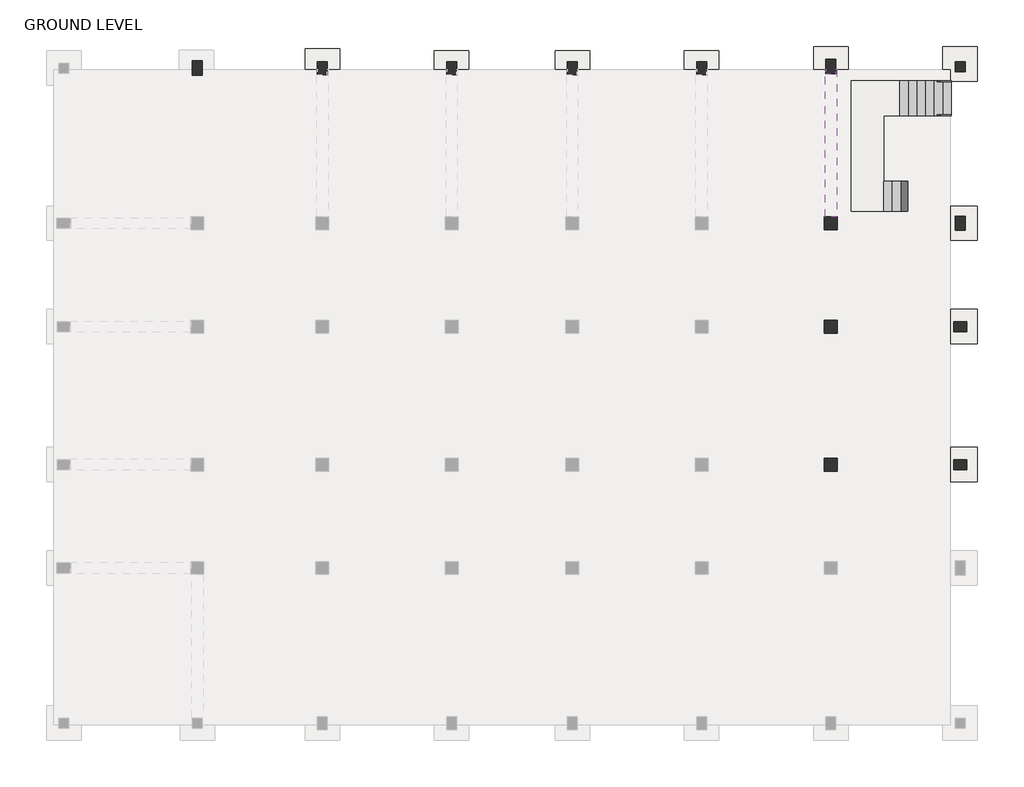
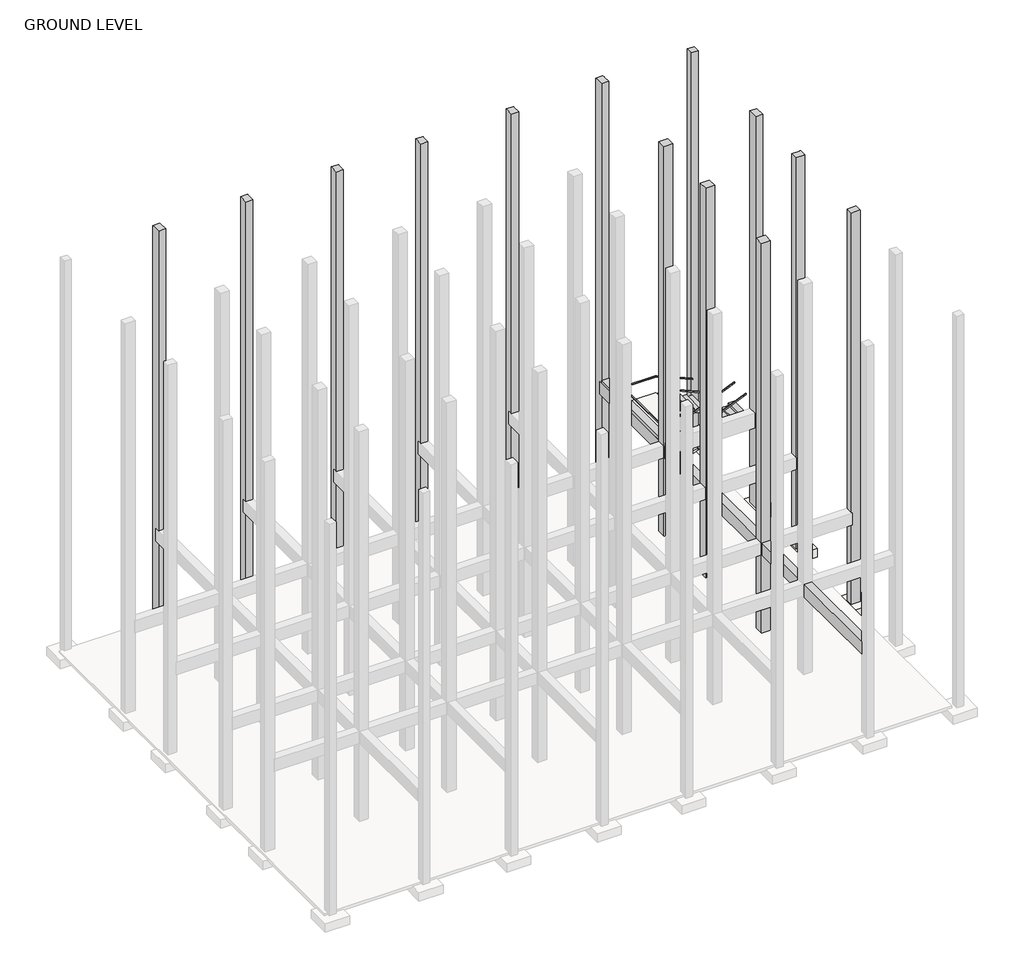
# One storey, part 3 of 3: 13 columns, 13 slabs, 2 railings, 2 stair flights, 1 beam.
"""IFC4 building model written with IfcOpenShell, lengths in millimetres."""

from ifc_helpers import new_model, si_unit, frame, origin, place, context, project, spatial, polyline, outline, extrude, faceted_brep, element, save

model = new_model("IFC4")

# Units and contexts
model_context = context("Model", 3, world=origin())
ifc_project = project(units=[si_unit("LENGTHUNIT", "METRE", prefix="MILLI")], contexts=[model_context])

# Site, building, storey
site = spatial("IfcSite", under=ifc_project)
building = spatial("IfcBuilding", under=site)
storey = spatial("IfcBuildingStorey", under=building, Name="GROUND LEVEL", Elevation=-1404.4011518)

# Beam
placement = place(None, origin())
element("IfcBeam", 1, ObjectType="M_Concrete-Rectangular Beam : 400 x 800mm", at=placement, inside=storey, context=model_context, shape_type="Brep", body=[
    faceted_brep([(1425.6508981, -990.0309165, 114.4), (1425.6508981, -6047.8309165, 114.4), (1425.6508981, -6047.8309165, 762.0), (1425.6508981, -990.0309165, 762.0), (1803.4508981, -6019.2309165, 114.4), (1447.8508981, -6019.2309165, 114.4), (1447.8508981, -6047.8309165, 114.4), (1825.6508981, -990.0309165, 114.4), (1825.6508981, -6047.8309165, 114.4), (1803.4508981, -6047.8309165, 114.4), (1825.6508981, -990.0309165, 762.0), (1825.6508981, -6047.8309165, 762.0), (1803.4508981, -6047.8309165, 762.0), (1803.4508981, -6019.2309165, 762.0), (1447.8508981, -6019.2309165, 762.0), (1447.8508981, -6047.8309165, 762.0)], [[[0, 1, 2, 3]], [[4, 5, 6, 1, 0, 7, 8, 9]], [[8, 7, 10, 11]], [[4, 9, 12, 13]], [[6, 5, 14, 15]], [[5, 4, 13, 14]], [[7, 0, 3, 10]], [[1, 6, 15, 2]], [[9, 8, 11, 12]], [[3, 2, 15, 14, 13, 12, 11, 10]]]),
    faceted_brep([(1803.4508981, 16713.7690835, 114.4), (1803.4508981, 16713.7690835, 914.4), (1803.4508981, 16869.3690835, 914.4), (1803.4508981, 16869.3690835, 114.4), (1447.8508981, 16713.7690835, 114.4), (1447.8508981, 16713.7690835, 762.0), (1447.8508981, 16713.7690835, 914.4), (1447.8508981, 16869.3690835, 114.4), (1447.8508981, 16869.3690835, 762.0), (1425.6508981, 11659.1690835, 114.4), (1825.6508981, 11659.1690835, 114.4), (1825.6508981, 11659.1690835, 914.4), (1447.8508981, 11659.1690835, 914.4), (1447.8508981, 11659.1690835, 762.0), (1425.6508981, 11659.1690835, 762.0), (1825.6508981, 16869.3690835, 914.4), (1425.6508981, 16869.3690835, 114.4), (1425.6508981, 16869.3690835, 762.0), (1825.6508981, 16869.3690835, 114.4)], [[[0, 1, 2, 3]], [[1, 0, 4, 5, 6]], [[4, 7, 8, 5]], [[9, 10, 11, 12, 13, 14]], [[1, 6, 12, 11, 15, 2]], [[16, 9, 14, 17]], [[4, 0, 3, 18, 10, 9, 16, 7]], [[11, 10, 18, 15]], [[3, 2, 15, 18]], [[7, 16, 17, 8]], [[13, 5, 8, 17, 14]], [[5, 13, 12, 6]]]),
    faceted_brep([(1825.6508981, 11201.9690835, 114.4), (1425.6508981, 11201.9690835, 114.4), (1425.6508981, 11201.9690835, 762.0), (1447.8508981, 11201.9690835, 762.0), (1447.8508981, 11201.9690835, 914.4), (1825.6508981, 11201.9690835, 914.4), (1425.6508981, 8001.5690835, 114.4), (1825.6508981, 8001.5690835, 114.4), (1825.6508981, 8001.5690835, 762.0), (1425.6508981, 8001.5690835, 762.0), (1447.8508981, 11176.5690835, 914.4), (1825.6508981, 11176.5690835, 914.4), (1825.6508981, 11176.5690835, 762.0), (1447.8508981, 11176.5690835, 762.0)], [[[0, 1, 2, 3, 4, 5]], [[6, 7, 8, 9]], [[5, 4, 10, 11]], [[1, 6, 9, 2]], [[1, 0, 7, 6]], [[0, 5, 11, 12, 8, 7]], [[12, 13, 3, 2, 9, 8]], [[13, 10, 4, 3]], [[10, 13, 12, 11]]]),
    faceted_brep([(1825.6508981, 7544.3690835, 114.4), (1425.6508981, 7544.3690835, 114.4), (1425.6508981, 7544.3690835, 762.0), (1825.6508981, 7544.3690835, 762.0), (1425.6508981, 3124.7690835, 114.4), (1825.6508981, 3124.7690835, 114.4), (1825.6508981, 3124.7690835, 762.0), (1425.6508981, 3124.7690835, 762.0)], [[[0, 1, 2, 3]], [[4, 5, 6, 7]], [[1, 4, 7, 2]], [[1, 0, 5, 4]], [[5, 0, 3, 6]], [[3, 2, 7, 6]]]),
    faceted_brep([(1425.6508981, -532.8309165, 114.4), (1825.6508981, -532.8309165, 114.4), (1825.6508981, -532.8309165, 762.0), (1425.6508981, -532.8309165, 762.0), (1425.6508981, 2667.5690835, 114.4), (1425.6508981, 2667.5690835, 762.0), (1825.6508981, 2667.5690835, 114.4), (1825.6508981, 2667.5690835, 762.0)], [[[0, 1, 2, 3]], [[4, 0, 3, 5]], [[1, 0, 4, 6]], [[1, 6, 7, 2]], [[6, 4, 5, 7]], [[3, 2, 7, 5]]]),
])

# Columns
element("IfcColumn", 2, ObjectType="M_Concrete-Rectangular-Column : C1", at=placement, inside=storey, context=model_context, shape_type="SweptSolid", body=[
    extrude(outline(polyline([(6375.4508981, 17145.5690835), (6375.4508981, 16789.9690835), (6019.8508981, 16789.9690835), (6019.8508981, 17145.5690835), (6375.4508981, 17145.5690835)])), frame((0.0, 0.0, -4147.6011518), z_axis=(0.0, 0.0, 1.0), x_axis=(1.0, 0.0, 0.0)), (0.0, 0.0, 1.0), 20911.6011518),
])
element("IfcColumn", 3, ObjectType="M_Concrete-Rectangular-Column : C2", at=placement, inside=storey, context=model_context, shape_type="Brep", body=[
    faceted_brep([(-16179.7491019, 17145.5690835, -4147.6011518), (-16179.7491019, 16688.3690835, -4147.6011518), (-16535.3491019, 16688.3690835, -4147.6011518), (-16535.3491019, 17145.5690835, -4147.6011518), (-16179.7491019, 17145.5690835, 16764.0), (-16179.7491019, 17116.9690835, 16764.0), (-16179.7491019, 17094.7690835, 16764.0), (-16179.7491019, 16688.3690835, 16764.0), (-16179.7491019, 17145.5690835, 114.4), (-16179.7491019, 17145.5690835, 914.4), (-16535.3491019, 16688.3690835, 16764.0), (-16535.3491019, 17094.7690835, 16764.0), (-16535.3491019, 17116.9690835, 16764.0), (-16535.3491019, 17145.5690835, 16764.0), (-16535.3491019, 17145.5690835, 914.4), (-16535.3491019, 17145.5690835, 114.4)], [[[0, 1, 2, 3]], [[4, 5, 6, 7, 1, 0, 8, 9]], [[7, 10, 2, 1]], [[10, 11, 12, 13, 14, 15, 3, 2]], [[13, 4, 9, 8, 0, 3, 15, 14]], [[4, 13, 12, 11, 10, 7, 6, 5]]]),
])
element("IfcColumn", 4, ObjectType="M_Concrete-Rectangular-Column : C2", at=placement, inside=storey, context=model_context, shape_type="Brep", body=[
    faceted_brep([(-11607.7491019, 17145.5690835, -4147.6011518), (-11607.7491019, 16688.3690835, -4147.6011518), (-11963.3491019, 16688.3690835, -4147.6011518), (-11963.3491019, 17145.5690835, -4147.6011518), (-11607.7491019, 17145.5690835, 16764.0), (-11607.7491019, 17116.9690835, 16764.0), (-11607.7491019, 17094.7690835, 16764.0), (-11607.7491019, 16688.3690835, 16764.0), (-11607.7491019, 17145.5690835, 114.4), (-11607.7491019, 17145.5690835, 914.4), (-11963.3491019, 16688.3690835, 16764.0), (-11963.3491019, 17094.7690835, 16764.0), (-11963.3491019, 17116.9690835, 16764.0), (-11963.3491019, 17145.5690835, 16764.0), (-11963.3491019, 17145.5690835, 914.4), (-11963.3491019, 17145.5690835, 114.4)], [[[0, 1, 2, 3]], [[4, 5, 6, 7, 1, 0, 8, 9]], [[7, 10, 2, 1]], [[10, 11, 12, 13, 14, 15, 3, 2]], [[13, 4, 9, 8, 0, 3, 15, 14]], [[4, 13, 12, 11, 10, 7, 6, 5]]]),
])
element("IfcColumn", 5, ObjectType="M_Concrete-Rectangular-Column : C2", at=placement, inside=storey, context=model_context, shape_type="Brep", body=[
    faceted_brep([(-7340.5491019, 17145.5690835, -4147.6011518), (-7340.5491019, 16688.3690835, -4147.6011518), (-7696.1491019, 16688.3690835, -4147.6011518), (-7696.1491019, 17145.5690835, -4147.6011518), (-7340.5491019, 17145.5690835, 16764.0), (-7340.5491019, 17116.9690835, 16764.0), (-7340.5491019, 17094.7690835, 16764.0), (-7340.5491019, 16688.3690835, 16764.0), (-7340.5491019, 17145.5690835, 114.4), (-7340.5491019, 17145.5690835, 914.4), (-7696.1491019, 16688.3690835, 16764.0), (-7696.1491019, 17094.7690835, 16764.0), (-7696.1491019, 17116.9690835, 16764.0), (-7696.1491019, 17145.5690835, 16764.0), (-7696.1491019, 17145.5690835, 914.4), (-7696.1491019, 17145.5690835, 114.4)], [[[0, 1, 2, 3]], [[4, 5, 6, 7, 1, 0, 8, 9]], [[7, 10, 2, 1]], [[10, 11, 12, 13, 14, 15, 3, 2]], [[13, 4, 9, 8, 0, 3, 15, 14]], [[4, 13, 12, 11, 10, 7, 6, 5]]]),
])
element("IfcColumn", 6, ObjectType="M_Concrete-Rectangular-Column : C2", at=placement, inside=storey, context=model_context, shape_type="Brep", body=[
    faceted_brep([(-2768.5491019, 17145.5690835, -4147.6011518), (-2768.5491019, 16688.3690835, -4147.6011518), (-3124.1491019, 16688.3690835, -4147.6011518), (-3124.1491019, 17145.5690835, -4147.6011518), (-2768.5491019, 17145.5690835, 16764.0), (-2768.5491019, 17116.9690835, 16764.0), (-2768.5491019, 17094.7690835, 16764.0), (-2768.5491019, 16688.3690835, 16764.0), (-2768.5491019, 17145.5690835, 114.4), (-2768.5491019, 17145.5690835, 914.4), (-3124.1491019, 16688.3690835, 16764.0), (-3124.1491019, 17094.7690835, 16764.0), (-3124.1491019, 17116.9690835, 16764.0), (-3124.1491019, 17145.5690835, 16764.0), (-3124.1491019, 17145.5690835, 914.4), (-3124.1491019, 17145.5690835, 114.4)], [[[0, 1, 2, 3]], [[4, 5, 6, 7, 1, 0, 8, 9]], [[7, 10, 2, 1]], [[10, 11, 12, 13, 14, 15, 3, 2]], [[13, 4, 9, 8, 0, 3, 15, 14]], [[4, 13, 12, 11, 10, 7, 6, 5]]]),
])
element("IfcColumn", 7, ObjectType="M_Concrete-Rectangular-Column : C2", at=placement, inside=storey, context=model_context, shape_type="Brep", body=[
    faceted_brep([(5969.0508981, 7950.7690835, -4147.6011518), (6426.2508981, 7950.7690835, -4147.6011518), (6426.2508981, 7595.1690835, -4147.6011518), (5969.0508981, 7595.1690835, -4147.6011518), (5969.0508981, 7950.7690835, 16764.0), (6375.4508981, 7950.7690835, 16764.0), (6397.6508981, 7950.7690835, 16764.0), (6426.2508981, 7950.7690835, 16764.0), (6426.2508981, 7595.1690835, 16764.0), (6397.6508981, 7595.1690835, 16764.0), (6375.4508981, 7595.1690835, 16764.0), (5969.0508981, 7595.1690835, 16764.0)], [[[0, 1, 2, 3]], [[4, 5, 6, 7, 1, 0]], [[7, 8, 2, 1]], [[8, 9, 10, 11, 3, 2]], [[11, 4, 0, 3]], [[4, 11, 10, 9, 8, 7, 6, 5]]]),
])
element("IfcColumn", 8, ObjectType="M_Concrete-Rectangular-Column : C2", at=placement, inside=storey, context=model_context, shape_type="Brep", body=[
    faceted_brep([(5969.0508981, 3073.9690835, -4147.6011518), (6426.2508981, 3073.9690835, -4147.6011518), (6426.2508981, 2718.3690835, -4147.6011518), (5969.0508981, 2718.3690835, -4147.6011518), (5969.0508981, 3073.9690835, 16764.0), (6375.4508981, 3073.9690835, 16764.0), (6397.6508981, 3073.9690835, 16764.0), (6426.2508981, 3073.9690835, 16764.0), (6426.2508981, 2718.3690835, 16764.0), (6397.6508981, 2718.3690835, 16764.0), (6375.4508981, 2718.3690835, 16764.0), (5969.0508981, 2718.3690835, 16764.0)], [[[0, 1, 2, 3]], [[4, 5, 6, 7, 1, 0]], [[7, 8, 2, 1]], [[8, 9, 10, 11, 3, 2]], [[11, 4, 0, 3]], [[4, 11, 10, 9, 8, 7, 6, 5]]]),
])
element("IfcColumn", 9, ObjectType="M_Concrete-Rectangular-Column : C3", at=placement, inside=storey, context=model_context, shape_type="SweptSolid", body=[
    extrude(outline(polyline([(1854.2508981, 11659.1690835), (1854.2508981, 11201.9690835), (1397.0508981, 11201.9690835), (1397.0508981, 11659.1690835), (1854.2508981, 11659.1690835)])), frame((0.0, 0.0, -4147.6011518), z_axis=(0.0, 0.0, 1.0), x_axis=(1.0, 0.0, 0.0)), (0.0, 0.0, 1.0), 20911.6011518),
])
element("IfcColumn", 10, ObjectType="M_Concrete-Rectangular-Column : C3", at=placement, inside=storey, context=model_context, shape_type="SweptSolid", body=[
    extrude(outline(polyline([(1854.2508981, 8001.5690835), (1854.2508981, 7544.3690835), (1397.0508981, 7544.3690835), (1397.0508981, 8001.5690835), (1854.2508981, 8001.5690835)])), frame((0.0, 0.0, -4147.6011518), z_axis=(0.0, 0.0, 1.0), x_axis=(1.0, 0.0, 0.0)), (0.0, 0.0, 1.0), 20911.6011518),
])
element("IfcColumn", 11, ObjectType="M_Concrete-Rectangular-Column : C3", at=placement, inside=storey, context=model_context, shape_type="SweptSolid", body=[
    extrude(outline(polyline([(1854.2508981, 3124.7690835), (1854.2508981, 2667.5690835), (1397.0508981, 2667.5690835), (1397.0508981, 3124.7690835), (1854.2508981, 3124.7690835)])), frame((0.0, 0.0, -4147.6011518), z_axis=(0.0, 0.0, 1.0), x_axis=(1.0, 0.0, 0.0)), (0.0, 0.0, 1.0), 20911.6011518),
])
element("IfcColumn", 12, ObjectType="M_Concrete-Rectangular-Column : C4", at=placement, inside=storey, context=model_context, shape_type="Brep", body=[
    faceted_brep([(-20599.3491019, 17170.9690835, -4147.6011518), (-20599.3491019, 16662.9690835, -4147.6011518), (-20954.9491019, 16662.9690835, -4147.6011518), (-20954.9491019, 17170.9690835, -4147.6011518), (-20599.3491019, 17170.9690835, 16764.0), (-20599.3491019, 17116.9690835, 16764.0), (-20599.3491019, 17094.7690835, 16764.0), (-20599.3491019, 16662.9690835, 16764.0), (-20599.3491019, 17170.9690835, 114.4), (-20599.3491019, 17170.9690835, 914.4), (-20954.9491019, 16662.9690835, 16764.0), (-20954.9491019, 17094.7690835, 16764.0), (-20954.9491019, 17116.9690835, 16764.0), (-20954.9491019, 17170.9690835, 16764.0), (-20954.9491019, 17170.9690835, 914.4), (-20954.9491019, 17170.9690835, 114.4)], [[[0, 1, 2, 3]], [[4, 5, 6, 7, 1, 0, 8, 9]], [[7, 10, 2, 1]], [[10, 11, 12, 13, 14, 15, 3, 2]], [[13, 4, 9, 8, 0, 3, 15, 14]], [[4, 13, 12, 11, 10, 7, 6, 5]]]),
])
element("IfcColumn", 13, ObjectType="M_Concrete-Rectangular-Column : C4", at=placement, inside=storey, context=model_context, shape_type="Brep", body=[
    faceted_brep([(1803.4508981, 17221.7690835, -4147.6011518), (1803.4508981, 16713.7690835, -4147.6011518), (1447.8508981, 16713.7690835, -4147.6011518), (1447.8508981, 17221.7690835, -4147.6011518), (1803.4508981, 17221.7690835, 16764.0), (1803.4508981, 17116.9690835, 16764.0), (1803.4508981, 17094.7690835, 16764.0), (1803.4508981, 16713.7690835, 16764.0), (1803.4508981, 17221.7690835, 114.4), (1803.4508981, 17221.7690835, 914.4), (1447.8508981, 16713.7690835, 16764.0), (1447.8508981, 17094.7690835, 16764.0), (1447.8508981, 17116.9690835, 16764.0), (1447.8508981, 17221.7690835, 16764.0), (1447.8508981, 17221.7690835, 914.4), (1447.8508981, 17221.7690835, 114.4)], [[[0, 1, 2, 3]], [[4, 5, 6, 7, 1, 0, 8, 9]], [[7, 10, 2, 1]], [[10, 11, 12, 13, 14, 15, 3, 2]], [[13, 4, 9, 8, 0, 3, 15, 14]], [[4, 13, 12, 11, 10, 7, 6, 5]]]),
])
element("IfcColumn", 14, ObjectType="M_Concrete-Rectangular-Column : C4", at=placement, inside=storey, context=model_context, shape_type="Brep", body=[
    faceted_brep([(6375.4508981, 11684.5690835, -4147.6011518), (6375.4508981, 11176.5690835, -4147.6011518), (6019.8508981, 11176.5690835, -4147.6011518), (6019.8508981, 11684.5690835, -4147.6011518), (6375.4508981, 11684.5690835, 16764.0), (6375.4508981, 11176.5690835, 16764.0), (6375.4508981, 11176.5690835, 16611.6), (6375.4508981, 11176.5690835, 15964.0), (6375.4508981, 11176.5690835, 13563.6), (6375.4508981, 11176.5690835, 12916.0), (6375.4508981, 11176.5690835, 10515.6), (6375.4508981, 11176.5690835, 9868.0), (6375.4508981, 11176.5690835, 7467.6), (6375.4508981, 11176.5690835, 6820.0), (6375.4508981, 11176.5690835, 4419.6), (6375.4508981, 11176.5690835, 3772.0), (6375.4508981, 11176.5690835, 762.0), (6375.4508981, 11176.5690835, 114.4), (6375.4508981, 11684.5690835, 114.4), (6375.4508981, 11684.5690835, 914.4), (6375.4508981, 11684.5690835, 3772.0), (6375.4508981, 11684.5690835, 4572.0), (6375.4508981, 11684.5690835, 6820.0), (6375.4508981, 11684.5690835, 7620.0), (6375.4508981, 11684.5690835, 9868.0), (6375.4508981, 11684.5690835, 10668.0), (6375.4508981, 11684.5690835, 12916.0), (6375.4508981, 11684.5690835, 13716.0), (6375.4508981, 11684.5690835, 15964.0), (6375.4508981, 11684.5690835, 16611.6), (6019.8508981, 11176.5690835, 16764.0), (6019.8508981, 11176.5690835, 16611.6), (6019.8508981, 11176.5690835, 15964.0), (6019.8508981, 11176.5690835, 13716.0), (6019.8508981, 11176.5690835, 13563.6), (6019.8508981, 11176.5690835, 12916.0), (6019.8508981, 11176.5690835, 10668.0), (6019.8508981, 11176.5690835, 10515.6), (6019.8508981, 11176.5690835, 9868.0), (6019.8508981, 11176.5690835, 7620.0), (6019.8508981, 11176.5690835, 7467.6), (6019.8508981, 11176.5690835, 6820.0), (6019.8508981, 11176.5690835, 4572.0), (6019.8508981, 11176.5690835, 4419.6), (6019.8508981, 11176.5690835, 3772.0), (6019.8508981, 11176.5690835, 914.4), (6019.8508981, 11176.5690835, 762.0), (6019.8508981, 11176.5690835, 114.4), (6019.8508981, 11684.5690835, 16764.0), (6019.8508981, 11684.5690835, 16611.6), (6019.8508981, 11684.5690835, 15964.0), (6019.8508981, 11684.5690835, 13716.0), (6019.8508981, 11684.5690835, 12916.0), (6019.8508981, 11684.5690835, 10668.0), (6019.8508981, 11684.5690835, 9868.0), (6019.8508981, 11684.5690835, 7620.0), (6019.8508981, 11684.5690835, 6820.0), (6019.8508981, 11684.5690835, 4572.0), (6019.8508981, 11684.5690835, 3772.0), (6019.8508981, 11684.5690835, 914.4), (6019.8508981, 11684.5690835, 114.4)], [[[0, 1, 2, 3]], [[4, 5, 6, 7, 8, 9, 10, 11, 12, 13, 14, 15, 16, 17, 1, 0, 18, 19, 20, 21, 22, 23, 24, 25, 26, 27, 28, 29]], [[5, 30, 31, 32, 33, 34, 35, 36, 37, 38, 39, 40, 41, 42, 43, 44, 45, 46, 47, 2, 1, 17, 16, 15, 14, 13, 12, 11, 10, 9, 8, 7, 6]], [[30, 48, 49, 50, 51, 52, 53, 54, 55, 56, 57, 58, 59, 60, 3, 2, 47, 46, 45, 44, 43, 42, 41, 40, 39, 38, 37, 36, 35, 34, 33, 32, 31]], [[48, 4, 29, 28, 27, 26, 25, 24, 23, 22, 21, 20, 19, 18, 0, 3, 60, 59, 58, 57, 56, 55, 54, 53, 52, 51, 50, 49]], [[4, 48, 30, 5]]]),
])

# Railings
element("IfcRailing", 15, ObjectType="Handrail", at=placement, inside=storey, context=model_context, shape_type="Brep", body=[
    faceted_brep([(5878.2258195, 16426.305974, -359.8261518), (5878.2258195, 16426.305974, -415.0651705), (5878.2258195, 16477.105974, -415.0651705), (5878.2258195, 16477.105974, -359.8261518), (4049.4258195, 16426.305974, 421.2238482), (4039.0320197, 16426.305974, 370.4238482), (4039.0320197, 16477.105974, 370.4238482), (4049.4258195, 16477.105974, 421.2238482), (2398.4258195, 16426.305974, 421.2238482), (2398.4258195, 16426.305974, 370.4238482), (2347.6258195, 16477.105974, 370.4238482), (2347.6258195, 16477.105974, 421.2238482), (2398.4258195, 11896.1816424, 421.2238482), (2398.4258195, 11896.1816424, 370.4238482), (2347.6258195, 11845.3816424, 370.4238482), (2347.6258195, 11845.3816424, 421.2238482), (3188.2923097, 11896.1816424, 421.2238482), (3198.6861096, 11896.1816424, 370.4238482), (3198.6861096, 11845.3816424, 370.4238482), (3188.2923097, 11845.3816424, 421.2238482), (5931.4923097, 11896.1816424, 1592.7988482), (5931.4923097, 11845.3816424, 1592.7988482), (5931.4923097, 11845.3816424, 1537.5598295), (5931.4923097, 11896.1816424, 1537.5598295)], [[[0, 1, 2, 3]], [[1, 0, 4, 5]], [[2, 1, 5, 6]], [[3, 2, 6, 7]], [[0, 3, 7, 4]], [[5, 4, 8, 9]], [[6, 5, 9, 10]], [[7, 6, 10, 11]], [[4, 7, 11, 8]], [[9, 8, 12, 13]], [[10, 9, 13, 14]], [[11, 10, 14, 15]], [[8, 11, 15, 12]], [[13, 12, 16, 17]], [[14, 13, 17, 18]], [[15, 14, 18, 19]], [[12, 15, 19, 16]], [[20, 21, 22, 23]], [[17, 16, 20, 23]], [[18, 17, 23, 22]], [[19, 18, 22, 21]], [[16, 19, 21, 20]]]),
])
element("IfcRailing", 16, ObjectType="Handrail", at=placement, inside=storey, context=model_context, shape_type="Brep", body=[
    faceted_brep([(5878.2258195, 15223.6852874, -359.8261518), (5878.2258195, 15223.6852874, -415.0651705), (5878.2258195, 15274.4852874, -415.0651705), (5878.2258195, 15274.4852874, -359.8261518), (4049.4258195, 15223.6852874, 421.2238482), (4039.0320197, 15223.6852874, 370.4238482), (4039.0320197, 15274.4852874, 370.4238482), (4049.4258195, 15274.4852874, 421.2238482), (3493.0923097, 15223.6852874, 421.2238482), (3493.0923097, 15223.6852874, 370.4238482), (3442.2923097, 15274.4852874, 370.4238482), (3442.2923097, 15274.4852874, 421.2238482), (3493.0923097, 12985.9409784, 421.2238482), (3493.0923097, 12935.1409784, 370.4238482), (3442.2923097, 12935.1409784, 370.4238482), (3442.2923097, 12985.9409784, 421.2238482), (3493.0923097, 12985.9409784, 583.9425982), (3493.0923097, 12935.1409784, 533.1425982), (3442.2923097, 12935.1409784, 533.1425982), (3442.2923097, 12985.9409784, 583.9425982), (3493.0923097, 12909.7409784, 583.9425982), (3493.0923097, 12909.7409784, 533.1425982), (3442.2923097, 12858.9409784, 533.1425982), (3442.2923097, 12858.9409784, 583.9425982), (3569.2923097, 12909.7409784, 583.9425982), (3579.6861096, 12909.7409784, 533.1425982), (3579.6861096, 12858.9409784, 533.1425982), (3569.2923097, 12858.9409784, 583.9425982), (5931.4923097, 12909.7409784, 1592.7988482), (5931.4923097, 12858.9409784, 1592.7988482), (5931.4923097, 12858.9409784, 1537.5598295), (5931.4923097, 12909.7409784, 1537.5598295)], [[[0, 1, 2, 3]], [[1, 0, 4, 5]], [[2, 1, 5, 6]], [[3, 2, 6, 7]], [[0, 3, 7, 4]], [[5, 4, 8, 9]], [[6, 5, 9, 10]], [[7, 6, 10, 11]], [[4, 7, 11, 8]], [[9, 8, 12, 13]], [[10, 9, 13, 14]], [[11, 10, 14, 15]], [[8, 11, 15, 12]], [[13, 12, 16, 17]], [[14, 13, 17, 18]], [[15, 14, 18, 19]], [[12, 15, 19, 16]], [[17, 16, 20, 21]], [[18, 17, 21, 22]], [[19, 18, 22, 23]], [[16, 19, 23, 20]], [[21, 20, 24, 25]], [[22, 21, 25, 26]], [[23, 22, 26, 27]], [[20, 23, 27, 24]], [[28, 29, 30, 31]], [[25, 24, 28, 31]], [[26, 25, 31, 30]], [[27, 26, 30, 29]], [[24, 27, 29, 28]]]),
])

# Slabs
element("IfcSlab", 17, ObjectType="7\" Thickness", at=placement, inside=storey, context=model_context, shape_type="Brep", body=[
    faceted_brep([(4049.4258195, 16477.105974, -493.1761518), (4049.4258195, 15223.6852874, -493.1761518), (4030.3758195, 15223.6852874, -623.3511518), (4030.3758195, 16477.105974, -623.3511518), (2347.6258195, 16477.105974, -493.1761518), (2347.6258195, 11845.3816424, -493.1761518), (3257.5052912, 11845.3816424, -493.1761518), (3493.0923097, 11845.3816424, -493.1761518), (3512.1423097, 11845.3816424, -493.1761518), (3512.1423097, 12909.7409784, -493.1761518), (3493.0923097, 12909.7409784, -493.1761518), (3493.0923097, 15223.6852874, -493.1761518), (3980.212838, 15223.6852874, -493.1761518), (3980.212838, 16477.105974, -493.1761518), (4030.3758195, 15223.6852874, -692.3999252), (4030.3758195, 16477.105974, -692.3999252), (3980.212838, 16477.105974, -670.9761518), (2347.6258195, 16477.105974, -670.9761518), (2347.6258195, 11845.3816424, -670.9761518), (3257.5052912, 11845.3816424, -670.9761518), (3493.0923097, 11845.3816424, -570.3608627), (3512.1423097, 11845.3816424, -562.2249252), (3512.1423097, 12909.7409784, -562.2249252), (3493.0923097, 12909.7409784, -570.3608627), (3493.0923097, 12909.7409784, -670.9761518), (3493.0923097, 15223.6852874, -670.9761518), (3980.212838, 15223.6852874, -670.9761518), (3257.5052912, 12909.7409784, -670.9761518)], [[[0, 1, 2, 3]], [[4, 5, 6, 7, 8, 9, 10, 11, 12, 1, 0, 13]], [[3, 2, 14, 15]], [[0, 3, 15, 16, 17, 4, 13]], [[5, 4, 17, 18]], [[5, 18, 19, 20, 7, 6]], [[8, 7, 20, 21]], [[9, 8, 21, 22]], [[10, 9, 22, 23]], [[11, 10, 23, 24, 25]], [[2, 1, 12, 11, 25, 26, 14]], [[24, 27, 19, 18, 17, 16, 26, 25]], [[27, 24, 23]], [[26, 16, 15, 14]], [[19, 27, 23, 22, 21, 20]]]),
])
element("IfcSlab", 18, ObjectType="M_Footing-Rectangular : F 5", at=placement, inside=storey, context=model_context, shape_type="SweptSolid", body=[
    extrude(outline(polyline([(17602.7690835, -4597.6011518), (16383.5690835, -4597.6011518), (16383.5690835, -4197.8282159), (16861.9544764, -4197.8282159), (16861.9544764, -4147.6011518), (17602.7690835, -4147.6011518), (17602.7690835, -4597.6011518)])), frame((-16967.1491019, 0.0, 0.0), z_axis=(1.0, 0.0, 0.0), x_axis=(0.0, 1.0, 0.0)), (0.0, 0.0, 1.0), 1219.2),
])
element("IfcSlab", 19, ObjectType="M_Footing-Rectangular : F 5", at=placement, inside=storey, context=model_context, shape_type="SweptSolid", body=[
    extrude(outline(polyline([(17526.5690835, -4597.6011518), (16307.3690835, -4597.6011518), (16307.3690835, -4197.8282159), (16861.9544764, -4197.8282159), (16861.9544764, -4147.6011518), (17526.5690835, -4147.6011518), (17526.5690835, -4597.6011518)])), frame((-12395.1491019, 0.0, 0.0), z_axis=(1.0, 0.0, 0.0), x_axis=(0.0, 1.0, 0.0)), (0.0, 0.0, 1.0), 1219.2),
])
element("IfcSlab", 20, ObjectType="M_Footing-Rectangular : F 5", at=placement, inside=storey, context=model_context, shape_type="SweptSolid", body=[
    extrude(outline(polyline([(17526.5690835, -4597.6011518), (16307.3690835, -4597.6011518), (16307.3690835, -4197.8282159), (16861.9544764, -4197.8282159), (16861.9544764, -4147.6011518), (17526.5690835, -4147.6011518), (17526.5690835, -4597.6011518)])), frame((-8127.9491019, 0.0, 0.0), z_axis=(1.0, 0.0, 0.0), x_axis=(0.0, 1.0, 0.0)), (0.0, 0.0, 1.0), 1219.2),
])
element("IfcSlab", 21, ObjectType="M_Footing-Rectangular : F 5", at=placement, inside=storey, context=model_context, shape_type="SweptSolid", body=[
    extrude(outline(polyline([(17526.5690835, -4597.6011518), (16307.3690835, -4597.6011518), (16307.3690835, -4197.8282159), (16861.9544764, -4197.8282159), (16861.9544764, -4147.6011518), (17526.5690835, -4147.6011518), (17526.5690835, -4597.6011518)])), frame((-3555.9491019, 0.0, 0.0), z_axis=(1.0, 0.0, 0.0), x_axis=(0.0, 1.0, 0.0)), (0.0, 0.0, 1.0), 1219.2),
])
element("IfcSlab", 22, ObjectType="M_Footing-Rectangular : F 5", at=placement, inside=storey, context=model_context, shape_type="SweptSolid", body=[
    extrude(outline(polyline([(17678.9690835, -4597.6011518), (16459.7690835, -4597.6011518), (16459.7690835, -4197.8282159), (16861.9544764, -4197.8282159), (16861.9544764, -4147.6011518), (17678.9690835, -4147.6011518), (17678.9690835, -4597.6011518)])), frame((1016.0508981, 0.0, 0.0), z_axis=(1.0, 0.0, 0.0), x_axis=(0.0, 1.0, 0.0)), (0.0, 0.0, 1.0), 1219.2),
])
element("IfcSlab", 23, ObjectType="M_Footing-Rectangular : F 5", at=placement, inside=storey, context=model_context, shape_type="Brep", body=[
    faceted_brep([(6807.2508981, 17678.9690835, -4147.6011518), (5588.0508981, 17678.9690835, -4147.6011518), (5588.0508981, 16861.9544764, -4147.6011518), (5842.0508981, 16861.9544764, -4147.6011518), (5842.0508981, 16459.7690835, -4147.6011518), (6807.2508981, 16459.7690835, -4147.6011518), (6807.2508981, 17678.9690835, -4597.6011518), (6807.2508981, 16459.7690835, -4597.6011518), (5588.0508981, 16459.7690835, -4597.6011518), (5588.0508981, 17678.9690835, -4597.6011518), (5588.0508981, 16459.7690835, -4197.8282159), (5588.0508981, 16861.9544764, -4197.8282159), (5842.0508981, 16459.7690835, -4197.8282159), (5842.0508981, 16861.9544764, -4197.8282159)], [[[0, 1, 2, 3, 4, 5]], [[6, 7, 8, 9]], [[1, 0, 6, 9]], [[9, 8, 10, 11, 2, 1]], [[8, 7, 5, 4, 12, 10]], [[0, 5, 7, 6]], [[13, 11, 10, 12]], [[13, 12, 4, 3]], [[11, 13, 3, 2]]]),
])
element("IfcSlab", 24, ObjectType="M_Footing-Rectangular : F 5", at=placement, inside=storey, context=model_context, shape_type="SweptSolid", body=[
    extrude(outline(polyline([(-4597.6011518, 5588.0508981), (-4597.6011518, 6807.2508981), (-4147.6011518, 6807.2508981), (-4147.6011518, 5842.0508981), (-4197.8282159, 5842.0508981), (-4197.8282159, 5588.0508981), (-4597.6011518, 5588.0508981)])), frame((0.0, 10820.9690835, 0.0), z_axis=(0.0, 1.0, 0.0), x_axis=(0.0, 0.0, 1.0)), (0.0, 0.0, 1.0), 1219.2),
])
element("IfcSlab", 25, ObjectType="M_Footing-Rectangular : F 5", at=placement, inside=storey, context=model_context, shape_type="SweptSolid", body=[
    extrude(outline(polyline([(2235.2508981, 12040.1690835), (2235.2508981, 10820.9690835), (1016.0508981, 10820.9690835), (1016.0508981, 12040.1690835), (2235.2508981, 12040.1690835)])), frame((0.0, 0.0, -4597.6011518), z_axis=(0.0, 0.0, 1.0), x_axis=(1.0, 0.0, 0.0)), (0.0, 0.0, 1.0), 399.772936),
])
element("IfcSlab", 26, ObjectType="M_Footing-Rectangular : F 5", at=placement, inside=storey, context=model_context, shape_type="SweptSolid", body=[
    extrude(outline(polyline([(2235.2508981, 8382.5690835), (2235.2508981, 7163.3690835), (1016.0508981, 7163.3690835), (1016.0508981, 8382.5690835), (2235.2508981, 8382.5690835)])), frame((0.0, 0.0, -4597.6011518), z_axis=(0.0, 0.0, 1.0), x_axis=(1.0, 0.0, 0.0)), (0.0, 0.0, 1.0), 399.772936),
])
element("IfcSlab", 27, ObjectType="M_Footing-Rectangular : F 5", at=placement, inside=storey, context=model_context, shape_type="SweptSolid", body=[
    extrude(outline(polyline([(-4597.6011518, 5588.0508981), (-4597.6011518, 6807.2508981), (-4147.6011518, 6807.2508981), (-4147.6011518, 5842.0508981), (-4197.8282159, 5842.0508981), (-4197.8282159, 5588.0508981), (-4597.6011518, 5588.0508981)])), frame((0.0, 7163.3690835, 0.0), z_axis=(0.0, 1.0, 0.0), x_axis=(0.0, 0.0, 1.0)), (0.0, 0.0, 1.0), 1219.2),
])
element("IfcSlab", 28, ObjectType="M_Footing-Rectangular : F 5", at=placement, inside=storey, context=model_context, shape_type="SweptSolid", body=[
    extrude(outline(polyline([(-4597.6011518, 5588.0508981), (-4597.6011518, 6807.2508981), (-4147.6011518, 6807.2508981), (-4147.6011518, 5842.0508981), (-4197.8282159, 5842.0508981), (-4197.8282159, 5588.0508981), (-4597.6011518, 5588.0508981)])), frame((0.0, 2286.5690835, 0.0), z_axis=(0.0, 1.0, 0.0), x_axis=(0.0, 0.0, 1.0)), (0.0, 0.0, 1.0), 1219.2),
])
element("IfcSlab", 29, ObjectType="M_Footing-Rectangular : F 5", at=placement, inside=storey, context=model_context, shape_type="SweptSolid", body=[
    extrude(outline(polyline([(2235.2508981, 3505.7690835), (2235.2508981, 2286.5690835), (1016.0508981, 2286.5690835), (1016.0508981, 3505.7690835), (2235.2508981, 3505.7690835)])), frame((0.0, 0.0, -4597.6011518), z_axis=(0.0, 0.0, 1.0), x_axis=(1.0, 0.0, 0.0)), (0.0, 0.0, 1.0), 399.772936),
])

# Stair flights
element("IfcStairFlight", 30, ObjectType="3/4\" Nosing", at=placement, inside=storey, context=model_context, shape_type="Brep", body=[
    faceted_brep([(5878.2258195, 16477.105974, -1274.2261518), (5878.2258195, 15223.6852874, -1274.2261518), (5859.1758195, 15223.6852874, -1404.4011518), (5859.1758195, 16477.105974, -1404.4011518), (5554.3758195, 16477.105974, -1274.2261518), (5554.3758195, 15223.6852874, -1274.2261518), (5554.3758195, 15223.6852874, -1343.2749252), (5697.5006429, 15223.6852874, -1404.4011518), (5697.5006429, 16477.105974, -1404.4011518), (5554.3758195, 16477.105974, -1343.2749252), (5573.4258195, 15223.6852874, -1144.0511518), (5573.4258195, 16477.105974, -1144.0511518), (5249.5758195, 16477.105974, -1144.0511518), (5249.5758195, 15223.6852874, -1144.0511518), (5249.5758195, 15223.6852874, -1213.0999252), (5249.5758195, 16477.105974, -1213.0999252), (5268.6258195, 15223.6852874, -1013.8761518), (5268.6258195, 16477.105974, -1013.8761518), (4944.7758195, 16477.105974, -1013.8761518), (4944.7758195, 15223.6852874, -1013.8761518), (4944.7758195, 15223.6852874, -1082.9249252), (4944.7758195, 16477.105974, -1082.9249252), (4963.8258195, 15223.6852874, -883.7011518), (4963.8258195, 16477.105974, -883.7011518), (4639.9758195, 16477.105974, -883.7011518), (4639.9758195, 15223.6852874, -883.7011518), (4639.9758195, 15223.6852874, -952.7499252), (4639.9758195, 16477.105974, -952.7499252), (4659.0258195, 15223.6852874, -753.5261518), (4659.0258195, 16477.105974, -753.5261518), (4335.1758195, 16477.105974, -753.5261518), (4335.1758195, 15223.6852874, -753.5261518), (4335.1758195, 15223.6852874, -822.5749252), (4335.1758195, 16477.105974, -822.5749252), (4030.3758195, 15223.6852874, -623.3511518), (4049.4258195, 15223.6852874, -623.3511518), (4354.2258195, 15223.6852874, -623.3511518), (4354.2258195, 16477.105974, -623.3511518), (4049.4258195, 16477.105974, -623.3511518), (4030.3758195, 16477.105974, -623.3511518), (4030.3758195, 15223.6852874, -692.3999252), (4049.4258195, 15223.6852874, -700.5358627), (4049.4258195, 16477.105974, -700.5358627), (4030.3758195, 16477.105974, -692.3999252)], [[[0, 1, 2, 3]], [[1, 0, 4, 5]], [[1, 5, 6, 7, 2]], [[4, 0, 3, 8, 9]], [[10, 11, 12, 13]], [[10, 13, 14, 6, 5]], [[12, 11, 4, 9, 15]], [[5, 4, 11, 10]], [[16, 17, 18, 19]], [[16, 19, 20, 14, 13]], [[18, 17, 12, 15, 21]], [[13, 12, 17, 16]], [[22, 23, 24, 25]], [[22, 25, 26, 20, 19]], [[24, 23, 18, 21, 27]], [[19, 18, 23, 22]], [[28, 29, 30, 31]], [[28, 31, 32, 26, 25]], [[30, 29, 24, 27, 33]], [[25, 24, 29, 28]], [[34, 35, 36, 37, 38, 39]], [[35, 34, 40, 41]], [[38, 37, 30, 33, 42]], [[34, 39, 43, 40]], [[31, 30, 37, 36]], [[3, 2, 7, 8]], [[8, 7, 6, 14, 20, 26, 32, 41, 40, 43, 42, 33, 27, 21, 15, 9]], [[36, 35, 41, 32, 31]], [[39, 38, 42, 43]]]),
])
element("IfcStairFlight", 31, ObjectType="3/4\" Nosing", at=placement, inside=storey, context=model_context, shape_type="Brep", body=[
    faceted_brep([(3493.0923097, 11845.3816424, -363.0011518), (3493.0923097, 12909.7409784, -363.0011518), (3512.1423097, 12909.7409784, -493.1761518), (3512.1423097, 11845.3816424, -493.1761518), (3816.9423097, 11845.3816424, -363.0011518), (3816.9423097, 12909.7409784, -363.0011518), (3816.9423097, 12909.7409784, -432.0499252), (3512.1423097, 12909.7409784, -562.2249252), (3512.1423097, 11845.3816424, -562.2249252), (3816.9423097, 11845.3816424, -432.0499252), (3797.8923097, 12909.7409784, -232.8261518), (3797.8923097, 11845.3816424, -232.8261518), (4121.7423097, 11845.3816424, -232.8261518), (4121.7423097, 12909.7409784, -232.8261518), (4121.7423097, 12909.7409784, -301.8749252), (4121.7423097, 11845.3816424, -301.8749252), (4102.6923097, 12909.7409784, -102.6511518), (4102.6923097, 11845.3816424, -102.6511518), (4426.5423097, 11845.3816424, -102.6511518), (4426.5423097, 12909.7409784, -102.6511518), (4426.5423097, 12909.7409784, -171.6999252), (4426.5423097, 11845.3816424, -171.6999252), (4407.4923097, 12909.7409784, 27.5238482), (4407.4923097, 11845.3816424, 27.5238482), (4731.3423097, 11845.3816424, 27.5238482), (4731.3423097, 12909.7409784, 27.5238482), (4731.3423097, 12909.7409784, -41.5249252), (4731.3423097, 11845.3816424, -41.5249252), (4712.2923097, 12909.7409784, 157.6988482), (4712.2923097, 11845.3816424, 157.6988482), (5036.1423097, 11845.3816424, 157.6988482), (5036.1423097, 12909.7409784, 157.6988482), (5036.1423097, 12909.7409784, 88.6500748), (5036.1423097, 11845.3816424, 88.6500748), (5017.0923097, 12909.7409784, 287.8738482), (5017.0923097, 11845.3816424, 287.8738482), (5340.9423097, 11845.3816424, 287.8738482), (5340.9423097, 12909.7409784, 287.8738482), (5340.9423097, 12909.7409784, 218.8250748), (5340.9423097, 11845.3816424, 218.8250748), (5321.8923097, 12909.7409784, 418.0488482), (5321.8923097, 11845.3816424, 418.0488482), (5645.7423097, 11845.3816424, 418.0488482), (5645.7423097, 12909.7409784, 418.0488482), (5645.7423097, 12909.7409784, 349.0000748), (5645.7423097, 11845.3816424, 349.0000748), (5626.6923097, 12909.7409784, 548.2238482), (5626.6923097, 11845.3816424, 548.2238482), (5931.4923097, 11845.3816424, 548.2238482), (5931.4923097, 12909.7409784, 548.2238482), (5931.4923097, 12909.7409784, 471.0391373), (5931.4923097, 11845.3816424, 471.0391373)], [[[0, 1, 2, 3]], [[1, 0, 4, 5]], [[1, 5, 6, 7, 2]], [[3, 2, 7, 8]], [[4, 0, 3, 8, 9]], [[10, 11, 12, 13]], [[10, 13, 14, 6, 5]], [[12, 11, 4, 9, 15]], [[11, 10, 5, 4]], [[16, 17, 18, 19]], [[16, 19, 20, 14, 13]], [[18, 17, 12, 15, 21]], [[17, 16, 13, 12]], [[22, 23, 24, 25]], [[22, 25, 26, 20, 19]], [[24, 23, 18, 21, 27]], [[23, 22, 19, 18]], [[28, 29, 30, 31]], [[28, 31, 32, 26, 25]], [[30, 29, 24, 27, 33]], [[29, 28, 25, 24]], [[34, 35, 36, 37]], [[34, 37, 38, 32, 31]], [[36, 35, 30, 33, 39]], [[35, 34, 31, 30]], [[40, 41, 42, 43]], [[40, 43, 44, 38, 37]], [[42, 41, 36, 39, 45]], [[41, 40, 37, 36]], [[46, 47, 48, 49]], [[46, 49, 50, 44, 43]], [[48, 47, 42, 45, 51]], [[49, 48, 51, 50]], [[47, 46, 43, 42]], [[7, 6, 14, 20, 26, 32, 38, 44, 50, 51, 45, 39, 33, 27, 21, 15, 9, 8]]]),
])

save(model, "model.ifc")

# Revit data of these elements
# Type "M_Concrete-Rectangular Beam : 400 x 800mm"
#   Length [instance default] = 5' - 0"
#   b = 1' - 3.74803"
#   h = 2' - 7.49606"
#   Structural Material [instance default] = Concrete, Cast-in-Place gray
#   Assembly Code = ""
# Type "M_Concrete-Rectangular-Column : C1"
#   b = 1' - 2"
#   h = 1' - 2"
#   Structural Material [instance default] = Concrete, Cast-in-Place gray
# Type "M_Concrete-Rectangular-Column : C2"
#   b = 1' - 2"
#   h = 1' - 6"
#   Structural Material [instance default] = Concrete, Cast-in-Place gray
# Type "M_Concrete-Rectangular-Column : C3"
#   b = 1' - 6"
#   h = 1' - 6"
#   Structural Material [instance default] = Concrete, Cast-in-Place gray
# Type "M_Concrete-Rectangular-Column : C4"
#   b = 1' - 2"
#   h = 1' - 8"
#   Structural Material [instance default] = Concrete, Cast-in-Place gray
# Type "Handrail"
#   Assembly Code = "C2010400"
#   built-in parameter 1008612 = 0.0416667 (stored number, unit not read)
#   built-in parameter 1008611 = 0.0416667 (stored number, unit not read)
#   built-in parameter 1008609 = 0.333333 (stored number, unit not read)
#   built-in parameter 1008604 = 0.166667 (stored number, unit not read)
#   built-in parameter 1008603 = 0.166667 (stored number, unit not read)
#   Railing Height = 3' - 0"
#   built-in parameter 1008630 = 2
#   built-in parameter 1008610 = 2
#   built-in parameter 1008618 = Baluster - Square : 3/4"
# Type "M_Footing-Rectangular : F 5"
#   Width = 4' - 0"
#   Length = 4' - 0"
#   Thickness = 1' - 5.71654"
#   Structural Material [instance default] = Concrete, Cast-in-Place gray
#   Assembly Code = ""
# Element 1 (IfcBeam, "M_Concrete-Rectangular Beam : 400 x 800mm")
#   Comments = ""
#   Structural Material = Concrete, Cast-in-Place gray
#   Phase Created = New Construction
#   Materials on its faces: "Concrete, Cast-in-Place gray"
# Element 2 (IfcColumn, "M_Concrete-Rectangular-Column : C1")
#   Comments = ""
#   Structural Material = Concrete, Cast-in-Place gray
#   Phase Created = New Construction
#   Materials on its faces: "Concrete, Cast-in-Place gray"
# Elements 3, 4, 5, 6, 7, 8 (IfcColumn, "M_Concrete-Rectangular-Column : C2")
#   Comments = ""
#   Structural Material = Concrete, Cast-in-Place gray
#   Phase Created = New Construction
#   Materials on its faces: "Concrete, Cast-in-Place gray"
# Elements 9, 10, 11 (IfcColumn, "M_Concrete-Rectangular-Column : C3")
#   Comments = ""
#   Structural Material = Concrete, Cast-in-Place gray
#   Phase Created = New Construction
#   Materials on its faces: "Concrete, Cast-in-Place gray"
# Elements 12, 13, 14 (IfcColumn, "M_Concrete-Rectangular-Column : C4")
#   Comments = ""
#   Structural Material = Concrete, Cast-in-Place gray
#   Phase Created = New Construction
#   Materials on its faces: "Concrete, Cast-in-Place gray"
# Elements 15, 16 (IfcRailing, "Handrail")
#   Phase Created = New Construction
# Element 17 (IfcSlab, "7\" Thickness")
#   Phase Created = New Construction
#   Materials on its faces: "Concrete, Cast-in-Place gray"
# Elements 18, 19, 20, 21, 22, 23, 24, 25, 26, 27, 28, 29 (IfcSlab, "M_Footing-Rectangular : F 5")
#   Comments = ""
#   Structural Material = Concrete, Cast-in-Place gray
#   Phase Created = New Construction
#   Materials on its faces: "Concrete, Cast-in-Place gray"
# Elements 30, 31 (IfcStairFlight, "3/4\" Nosing")
#   Phase Created = New Construction
#   Materials on its faces: "Concrete, Cast-in-Place gray"
# Materials
#   "Concrete, Cast-in-Place gray": class "Concrete", colour RGB 192 192 192, transparency 0, Description = "Cast-in-place concrete", Cost = 0
